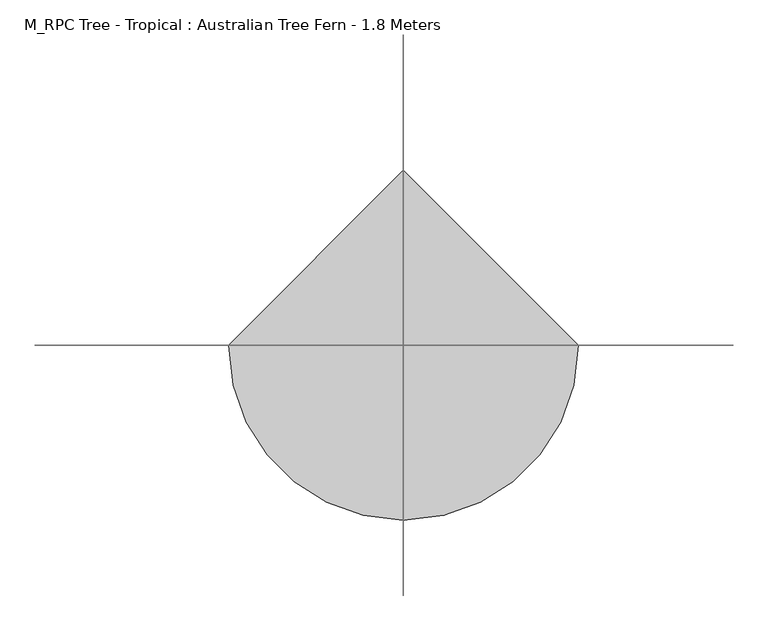
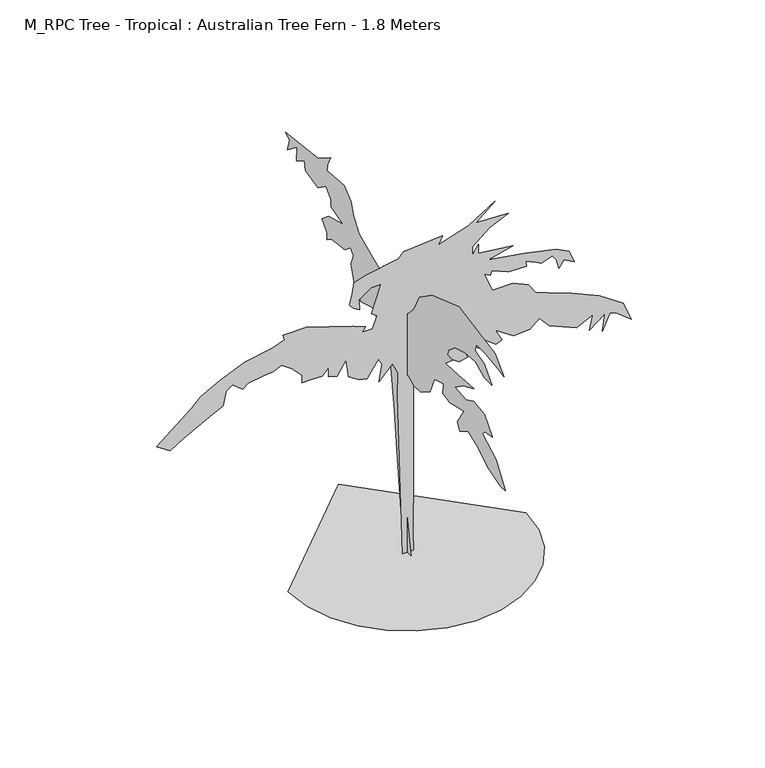
"""IFC4 building model written with IfcOpenShell, lengths in millimetres: geographic element geometry, M_RPC Tree - Tropical : Australian Tree Fern - 1.8 Meters."""

from ifc_helpers import new_model, si_unit, origin, place, context, project, spatial, triangles, source, transform, mapped, element, save


def m_rpc_tree_tropical_australian_tree_fern_1_8_meters_0203a3dd(model_context):
    return source(origin(), model_context, "Body", "Tessellation", [
        triangles([(-628.7763731, 0.0, 0.0007046), (-612.1463562, -144.1188648, 0.0007046), (-564.7912525, -276.4677177, 0.0007046), (-490.4986942, -393.2578274, 0.0007046), (-393.0611461, -490.6953755, 0.0007046), (-276.2710546, -564.9879338, 0.0007046), (-143.9221926, -612.3430012, 0.0007046), (0.1966986, -628.9730181, 0.0007046), (144.3155371, -612.345472, 0.0007046), (276.6643809, -564.9879338, 0.0007046), (393.4545087, -490.6953755, 0.0007046), (490.8920568, -393.2578274, 0.0007046), (565.1846151, -276.4677177, 0.0007046), (612.5396461, -144.1188648, 0.0007046), (629.169663, 5.5e-05, 0.0007046), (0.1965886, 628.9730181, 0.0007046), (463.0895388, -3.44e-05, 1800.0014671), (362.9519737, -2.93e-05, 1714.1689156), (534.6171132, -2.89e-05, 1707.0162998), (434.4795118, -2.61e-05, 1660.5237888), (345.0694533, -2.17e-05, 1585.4212509), (345.0694533, -1.89e-05, 1538.9287399), (377.2569872, -2.19e-05, 1588.9963234), (377.2569872, -1.89e-05, 1538.9287399), (559.6521403, -1.76e-05, 1517.4711834), (430.9020412, -1.57e-05, 1485.2837585), (624.0246283, -1.38e-05, 1453.0961884), (788.537261, -1.16e-05, 1417.333691), (856.4873285, -9.5e-06, 1381.5685776), (885.0973555, -5.5e-06, 1313.6185101), (827.8773016, -7.4e-06, 1345.8060802), (802.8422745, -5e-06, 1306.4660397), (788.537261, -8.2e-06, 1360.111021), (767.0797771, -9.9e-06, 1388.721048), (709.8571798, -8.7e-06, 1367.2636368), (681.2472256, -9.5e-06, 1381.5685776), (627.6021715, -1.1e-05, 1406.6036774), (631.1771713, -9.3e-06, 1377.9936504), (588.2621673, -9.3e-06, 1377.9936504), (534.6171132, -9.5e-06, 1381.5685776), (445.2095255, -1.16e-05, 1417.333691), (441.6320186, -1.01e-05, 1392.2985912), (409.444521, -1.12e-05, 1410.1810753), (452.3620322, -5e-06, 1306.4660397), (559.6521403, -5e-06, 1306.4660397), (641.907185, -2.9e-06, 1270.7035423), (677.6696823, 3e-07, 1217.0584883), (742.04475, 1.8e-06, 1192.0234612), (870.792342, 4.8e-06, 1141.9534069), (1017.4224907, 8.6e-06, 1077.5808826), (1142.5950829, 1.37e-05, 991.7482584), (1185.5101233, 1.99e-05, 888.0332228), (1103.2550423, 1.61e-05, 952.4082905), (1071.0674721, 1.56e-05, 959.5607609), (1031.7275042, 2.08e-05, 873.7282093), (1046.0325176, 1.52e-05, 966.7133039), (963.7774366, 1.91e-05, 902.340707), (981.6599207, 1.42e-05, 984.595788), (895.8273691, 1.67e-05, 941.6782768), (752.7747637, 1.31e-05, 1002.4782721), (699.1297096, 9.5e-06, 1063.2758692), (649.0596554, 1.2e-05, 1020.3582853), (563.2271401, 1.24e-05, 1013.2058149), (466.6670457, 8.6e-06, 1077.5808826), (502.4295794, 1.24e-05, 1013.2058149), (470.2420455, 1.33e-05, 998.9008015), (320.0369333, 6.5e-06, 1113.34338), (413.022028, 1.42e-05, 984.595788), (280.6968927, 8.6e-06, 1077.5808826), (320.0369333, 1.46e-05, 977.4433176), (273.544386, 1.5e-05, 970.2907745), (187.7115619, 1.14e-05, 1031.088299), (87.5742421, 9.5e-06, 1063.2758692), (191.2880696, 1.5e-05, 970.2907745), (30.352694, 1.1e-05, 1038.2408421), (33.9289474, 1.54e-05, 963.1383041), (33.9289474, 3.27e-05, 673.4530066), (33.9289474, 4.76e-05, 423.1103293), (30.352694, 6.66e-05, 104.8153318), (33.9289474, 7.24e-05, 0.0013067), (-23.2925485, 7.27e-05, 0.0006893), (-51.903368, 1.95e-05, 895.1882366), (-48.3268649, 1.2e-05, 1020.3582853), (-76.9376367, 8.4e-06, 1081.1558825), (-148.4644481, 1.29e-05, 1006.0532719), (-134.1591893, 7.3e-06, 1099.0383665), (-152.0409467, 5.4e-06, 1131.2259367), (-180.6514732, 7.8e-06, 1091.8858961), (-212.8384984, 1.05e-05, 1045.3933125), (-252.178539, 1.01e-05, 1052.5458555), (-309.4010636, 8e-06, 1088.3083529), (-323.7060771, 2e-06, 1188.4459179), (-370.1986244, 6.5e-06, 1113.34338), (-416.6911354, 5.6e-06, 1127.6483934), (-416.6911354, 2.6e-06, 1177.7184477), (-448.8761621, 4.8e-06, 1141.9534069), (-509.6737229, 4.8e-06, 1141.9534069), (-556.1662703, 4.8e-06, 1141.9534069), (-556.1662703, 2.2e-06, 1184.8709181), (-609.8138678, -1e-06, 1238.5159721), (-663.4563784, -3.3e-06, 1277.8560127), (-709.9488894, -2e-06, 1256.3984562), (-760.0189436, -1.8e-06, 1252.8210583), (-842.2740246, -1e-06, 1238.5159721), (-870.8865223, 3e-07, 1217.0584883), (-924.5315763, -2.3e-06, 1259.9735287), (-956.7166031, -8e-07, 1234.9384289), (-974.5991598, 3.7e-06, 1159.8359636), (-1074.7367249, 6.7e-06, 1109.7683802), (-1185.6043036, 1.03e-05, 1048.9708557), (-1253.5542984, 1.29e-05, 1006.0532719), (-1325.0819092, 1.01e-05, 1052.5458555), (-1139.1117926, 1.2e-06, 1202.7534748), (-1092.6192089, -1.8e-06, 1252.8210583), (-992.4816439, -5e-06, 1306.4660397), (-860.1565086, -8.4e-06, 1363.6885643), (-709.9488894, -1.01e-05, 1392.2985912), (-649.1513649, -1.14e-05, 1413.7561478), (-656.303908, -1.31e-05, 1442.3661747), (-531.1337502, -1.31e-05, 1442.3661747), (-409.5361579, -1.08e-05, 1403.0286049), (-287.9410727, -8.4e-06, 1363.6885643), (-219.9912595, -6.9e-06, 1338.6536098), (-237.873035, -5.5e-06, 1313.6185101), (-184.2277266, -5.5e-06, 1313.6185101), (-159.1934625, -9.3e-06, 1377.9936504), (-187.8042343, -1.06e-05, 1399.4510616), (-137.7354336, -1.93e-05, 1546.0812103), (-191.3804877, -1.93e-05, 1546.0812103), (-255.7535388, -1.65e-05, 1499.5886993), (-252.178539, -1.31e-05, 1442.3661747), (-284.3660728, -1.44e-05, 1463.826202), (-305.8235567, -1.59e-05, 1488.8586857), (-291.5185614, -1.91e-05, 1542.5036671), (-280.7885659, -2.27e-05, 1603.303735), (-216.4150061, -2.4e-05, 1624.7612915), (-44.7506115, -2.59e-05, 1656.9488617), (-19.7161203, -2.76e-05, 1685.5588886), (187.7115619, -2.87e-05, 1703.4413727), (166.2535512, -2.61e-05, 1660.5237888), (323.6119331, -2.91e-05, 1710.5938431), (0.1967009, -848.2856489, 1525.4262211), (0.1966947, -721.9905962, 1545.7961987), (0.1966909, -636.4380421, 1545.7961987), (0.1966914, -620.1404903, 1505.0562435), (0.1966961, -709.7680864, 1480.611224), (0.1967013, -774.9531338, 1403.206065), (0.1966982, -705.6955879, 1403.206065), (0.1966934, -624.2155323, 1443.9461655), (0.1966894, -530.5129306, 1435.7960815), (0.1966861, -436.812836, 1407.2786362), (0.196685, -379.7777999, 1358.3910679), (0.1966854, -367.5552901, 1325.7985806), (0.1966876, -416.4428221, 1325.7985806), (0.1966864, -351.2577747, 1268.7635445), (0.1966897, -428.6653318, 1272.8385864), (0.1966975, -611.9930225, 1285.0610962), (0.1966943, -510.1429167, 1240.2459538), (0.1966926, -436.812836, 1187.2834162), (0.1966974, -538.6629418, 1179.1359484), (0.1966995, -607.9204877, 1211.7284357), (0.1967043, -705.6955879, 1199.5059259), (0.1967102, -783.1006016, 1118.0258703), (0.1967074, -713.8430557, 1105.805904), (0.1967071, -689.4005796, 1081.3608845), (0.1967146, -811.6181196, 1012.1033386), (0.1967223, -901.2457157, 889.8831825), (0.1967202, -852.3581474, 885.810684), (0.1967138, -734.213106, 922.4757425), (0.1967074, -632.3630001, 983.5858206), (0.1967032, -559.0329557, 1016.1783079), (0.1967012, -481.6253986, 967.2882689), (0.1966991, -461.2553847, 1008.0282967), (0.1966989, -522.3654264, 1105.805904), (0.196694, -391.9978025, 1073.213344), (0.1966907, -326.8152623, 1085.4358538), (0.1966892, -330.8877608, 1142.4708899), (0.1966863, -249.4091949, 1118.0258703), (0.1966873, -208.6694215, 1024.3258484), (0.1966852, -127.189602, 971.3633108), (0.1966824, -62.006049, 967.2882689), (0.1966794, -13.1181855, 995.8083303), (0.1966778, 31.6955263, 983.5858206), (0.1966755, 52.0655402, 1028.3983469), (0.1966759, 80.5833171, 971.3633108), (0.1966779, 84.6573144, 898.030723), (0.1966865, 56.1395466, 653.5930269), (0.1966983, 19.473666, 311.3777598), (0.1967098, -33.4880268, 0.0007036), (0.1967069, 35.7695282, 0.0), (0.1967013, 52.0655402, 164.7148733), (0.1966905, 88.7315752, 470.2628654), (0.1966817, 117.2490932, 722.8505728), (0.1966725, 153.9151146, 975.4382801), (0.1966664, 206.8769073, 1101.730862), (0.1966639, 263.9127065, 1101.730862), (0.1966599, 300.5777468, 1179.1359484), (0.1966575, 365.762776, 1162.8409401), (0.1966555, 422.7978484, 1142.4708899), (0.196651, 483.9078901, 1203.5809679), (0.1966468, 512.4254082, 1301.3560318), (0.196646, 492.0553943, 1358.3910679), (0.1966439, 520.5729123, 1386.9086586), (0.1966429, 569.4604443, 1346.1685581), (0.1966379, 691.6805277, 1329.8736225), (0.196637, 732.4205555, 1301.3560318), (0.1966357, 732.4205555, 1342.0961323), (0.1966321, 781.3081238, 1390.9835552), (0.1966334, 720.1980457, 1439.8711235), (0.1966381, 589.8304582, 1476.536182), (0.1966324, 695.7555696, 1509.1286694), (0.1966311, 699.8280682, 1545.7961987), (0.1966277, 744.6430653, 1594.6837669), (0.196626, 817.9731823, 1541.721302), (0.1966201, 932.0457253, 1566.1637054), (0.1966183, 940.1932657, 1615.0537445), (0.1966162, 1013.5257809, 1574.3137894), (0.1966141, 1009.4508116, 1651.718803), (0.1966123, 1095.0059092, 1586.5338284), (0.1966112, 1078.7083574, 1647.6437611), (0.1966088, 1115.3758867, 1672.0887806), (0.1966211, 817.9731823, 1704.6814133), (0.196624, 703.9030375, 1778.011385), (0.1966245, 728.3455862, 1725.0513908), (0.1966254, 736.4955975, 1684.3112904), (0.196632, 577.6079484, 1700.6063713), (0.1966365, 512.4254082, 1647.6437611), (0.1966393, 492.0553943, 1582.4612572), (0.1966437, 439.0928567, 1513.2037113), (0.1966509, 316.875244, 1456.1662045), (0.1966608, 141.6931136, 1386.9086586), (0.1966549, 223.1726787, 1464.316143), (0.1966615, 113.1750868, 1407.2786362), (0.1966689, -0.8962257, 1329.8736225), (0.1966697, -62.006049, 1395.0585972), (0.1966689, -110.8938398, 1492.8337337), (0.1966718, -229.039181, 1574.3137894), (0.1966802, -473.4778945, 1659.8662708), (0.196691, -689.4005796, 1619.1263157), (0.1966968, -803.4706518, 1598.7563381), (0.1967028, -884.9507074, 1517.2762825)], [[15, 16, 1], [14, 15, 1], [14, 1, 2], [13, 14, 2], [13, 2, 3], [13, 3, 4], [12, 13, 4], [11, 12, 4], [11, 4, 5], [11, 5, 6], [11, 6, 7], [11, 7, 8], [11, 8, 9], [11, 9, 10], [141, 17, 18], [54, 55, 56], [73, 74, 75], [67, 68, 69], [24, 25, 26], [18, 19, 20], [51, 52, 53], [22, 23, 24], [84, 85, 86], [29, 30, 31], [56, 57, 58], [31, 32, 33], [130, 131, 132], [138, 139, 140], [41, 42, 43], [111, 112, 113], [110, 111, 113], [109, 110, 113], [122, 123, 124], [118, 119, 120], [18, 20, 21], [141, 18, 21], [69, 70, 71], [69, 71, 72], [28, 29, 31], [28, 31, 33], [28, 33, 34], [27, 28, 34], [27, 34, 35], [27, 35, 36], [27, 36, 37], [130, 132, 133], [130, 133, 134], [50, 51, 53], [50, 53, 54], [50, 54, 56], [50, 56, 58], [140, 141, 21], [37, 38, 39], [64, 65, 66], [64, 66, 67], [80, 81, 82], [79, 80, 82], [78, 79, 82], [77, 78, 82], [76, 77, 82], [76, 82, 83], [75, 76, 83], [97, 98, 99], [49, 50, 58], [49, 58, 59], [49, 59, 60], [48, 49, 60], [48, 60, 61], [47, 48, 61], [129, 130, 134], [129, 134, 135], [129, 135, 136], [129, 136, 137], [128, 129, 137], [108, 109, 113], [108, 113, 114], [107, 108, 114], [107, 114, 115], [106, 107, 115], [106, 115, 116], [105, 106, 116], [104, 105, 116], [103, 104, 116], [103, 116, 117], [102, 103, 117], [101, 102, 117], [101, 117, 118], [75, 83, 84], [26, 27, 37], [26, 37, 39], [26, 39, 40], [26, 40, 41], [26, 41, 43], [92, 93, 94], [92, 94, 95], [126, 127, 128], [101, 118, 120], [100, 101, 120], [100, 120, 121], [99, 100, 121], [97, 99, 121], [96, 97, 121], [95, 96, 121], [95, 121, 122], [92, 95, 122], [92, 122, 124], [140, 21, 22], [88, 89, 90], [24, 26, 43], [22, 24, 43], [88, 90, 91], [88, 91, 92], [88, 92, 124], [87, 88, 124], [87, 124, 125], [47, 61, 62], [47, 62, 63], [47, 63, 64], [46, 47, 64], [45, 46, 64], [44, 45, 64], [44, 64, 67], [43, 44, 67], [137, 138, 140], [128, 137, 140], [126, 128, 140], [126, 140, 22], [126, 22, 43], [126, 43, 67], [126, 67, 69], [126, 69, 72], [126, 72, 73], [125, 126, 73], [87, 125, 73], [87, 73, 75], [87, 75, 84], [87, 84, 86], [231, 232, 233], [156, 157, 158], [240, 241, 142], [222, 223, 224], [218, 219, 220], [220, 221, 222], [218, 220, 222], [153, 154, 155], [240, 142, 143], [239, 240, 143], [146, 147, 148], [205, 206, 207], [162, 163, 164], [156, 158, 159], [216, 217, 218], [216, 218, 222], [166, 167, 168], [166, 168, 169], [222, 224, 225], [239, 143, 144], [238, 239, 144], [146, 148, 149], [145, 146, 149], [165, 166, 169], [165, 169, 170], [207, 208, 209], [188, 189, 190], [188, 190, 191], [188, 191, 192], [187, 188, 192], [187, 192, 193], [186, 187, 193], [186, 193, 194], [185, 186, 194], [171, 172, 173], [171, 173, 174], [145, 149, 150], [155, 156, 159], [165, 170, 171], [165, 171, 174], [175, 176, 177], [182, 183, 184], [205, 207, 209], [205, 209, 210], [204, 205, 210], [203, 204, 210], [161, 162, 164], [161, 164, 165], [161, 165, 174], [160, 161, 174], [159, 160, 174], [159, 174, 175], [159, 175, 177], [155, 159, 177], [238, 144, 145], [238, 145, 150], [237, 238, 150], [237, 150, 151], [237, 151, 152], [236, 237, 152], [235, 236, 152], [235, 152, 153], [235, 153, 155], [235, 155, 177], [235, 177, 178], [234, 235, 178], [234, 178, 179], [234, 179, 180], [234, 180, 181], [234, 181, 182], [234, 182, 184], [231, 233, 234], [231, 234, 184], [214, 215, 216], [214, 216, 222], [213, 214, 222], [213, 222, 225], [213, 225, 226], [212, 213, 226], [212, 226, 227], [212, 227, 228], [211, 212, 228], [210, 211, 228], [210, 228, 229], [203, 210, 229], [203, 229, 230], [202, 203, 230], [184, 185, 194], [184, 194, 195], [231, 184, 195], [230, 231, 195], [230, 195, 196], [230, 196, 197], [202, 230, 197], [202, 197, 198], [201, 202, 198], [200, 201, 198], [199, 200, 198]], closed=False),
    ])


if __name__ == "__main__":
    model = new_model("IFC4")
    model_context = context("Model", 3, world=origin())
    ifc_project = project(units=[si_unit("LENGTHUNIT", "METRE", prefix="MILLI")], contexts=[model_context])
    site = spatial("IfcSite", under=ifc_project)
    building = spatial("IfcBuilding", under=site)
    placement = place(None, origin())
    m_rpc_tree_tropical_australian_tree_fern_1_8_meters_shape = m_rpc_tree_tropical_australian_tree_fern_1_8_meters_0203a3dd(model_context)
    element("IfcGeographicElement", 1, ObjectType="M_RPC Tree - Tropical : Australian Tree Fern - 1.8 Meters", at=placement, inside=building, context=model_context, shape_type="MappedRepresentation", body=[
        mapped(m_rpc_tree_tropical_australian_tree_fern_1_8_meters_shape, transform((0.0, 0.0, 0.0), x_axis=(1.0, 0.0, 0.0), y_axis=(0.0, 1.0, 0.0), z_axis=(0.0, 0.0, 1.0))),
    ])
    save(model, "model.ifc")

# Revit data of these elements
# Type "M_RPC Tree - Tropical : Australian Tree Fern - 1.8 Meters"
#   built-in parameter 1005198 = "{2, 15},{39, RPC-16-FVCN-UWG0-AP53-A000-ST1L-LVER-AU},{1, 0},{1, 0},{2, 35},{1, 8},{5, Color},{1, 0},{1, 0},{3, 0.8},{3, 0.8},{3, 0.8},{1, 8},{7, BBoxMin},{1, 0},{1, 0},{1, 0},{1, 0},{1, 0},{1, 8},{7, BBoxMax},{1, 0},{1, 0},{1, 0},{1, 0},{1, 0},{2, 11},{9, RPCTypeId},{1, 0},{1, 0},{39, RPC-16-FVCN-UWG0-AP53-A000-ST1L-LVER-AU},{1, 6},{14, RPCPlantHeight},{1, 0},{1, 0},{7, 5.90551},{2, 11},{7, keyword},{1, 0},{1, 0},{99, :Geometry:RPC:Australian Tree Fern:Alsophila cooperi (Cyathea australis):Sydney:Tree fern:Tropical.},{2, 11},{8, category},{1, 0},{1, 0},{17, :Trees [Tropical]},{2, 11},{12, LocalizedUID},{1, 0},{1, 0},{20, Australian Tree Fern},{2, 14},{6, Height},{1, 0},{1, 0},{7, 5.90551},{1, 2},{16, Cast Reflections},{1, 0},{1, 0},{1, 0},{1, 2},{12, Cast Shadows},{1, 0},{1, 0},{1, 1},{1, 2},{9, Lock View},{1, 0},{1, 0},{1, 0},{1, 4},{5, ViewC},{1, 0},{1, 0},{1, 0},{2, 11},{20, AdvancedUIDefinition},{1, 0},{1, 0},{0, },{2, 11},{10, AssetLibID},{1, 0},{1, 0},{36, 4D3F6E72-3F99-4203-98E9-AF80B3C7A7A4},{2, 11},{10, BaseSchema},{1, 0},{1, 0},{9, RPCSchema},{2, 11},{12, ExchangeGUID},{1, 0},{1, 0},{0, },{1, 2},{6, Hidden},{1, 0},{1, 0},{1, 0},{1, 4},{11, RPCCategory},{1, 0},{1, 0},{1, 0},{2, 11},{8, RPCImage},{1, 0},{1, 0},{0, },{1, 4},{13, SchemaVersion},{1, 0},{1, 0},{1, 4},{2, 11},{12, UIDefinition},{1, 0},{1, 0},{0, },{2, 11},{6, UIName},{1, 0},{1, 0},{39, RPC-16-FVCN-UWG0-AP53-A000-ST1L-LVER-AU},{2, 11},{11, VersionGUID},{1, 0},{1, 0},{9, RPCSchema},{2, 11},{9, assettype},{1, 0},{1, 0},{11, RPCGeometry},{2, 11},{11, description},{1, 0},{1, 0},{0, },{2, 11},{9, localname},{1, 0},{1, 0},{3, RPC},{2, 11},{9, localtype},{1, 0},{1, 0},{3, RPC},{1, 4},{8, revision},{1, 0},{1, 0},{1, 1},{2, 11},{9, thumbnail},{1, 0},{1, 0},{0, },{1, 4},{7, version},{1, 0},{1, 0},{1, 1},{1, 2},{20, RPC_Cast Reflections},{1, 0},{1, 0},{1, 1},{1, 2},{16, RPC_Cast Shadows},{1, 0},{1, 0},{1, 1},{1, 2},{13, RPC_Lock View},{1, 0},{1, 0},{1, 0},{1, 4},{9, RPC_ViewC},{1, 0},{1, 0},{1, 0},{21, assetlibrary_base.fbx},{1, 5},"
#   built-in parameter 1005195 = "RPC-16-FVCN-UWG0-AP53-A000-ST1L-LVER-AU"
#   Type Comments = "Australian Tree Fern"
#   Height = 5' - 10.86614"
#   Plan Symbol = element 411919
#   Description = (empty or 0)
#   Default Elevation = 0
